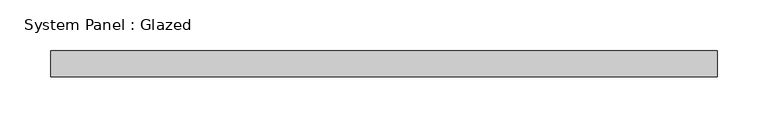
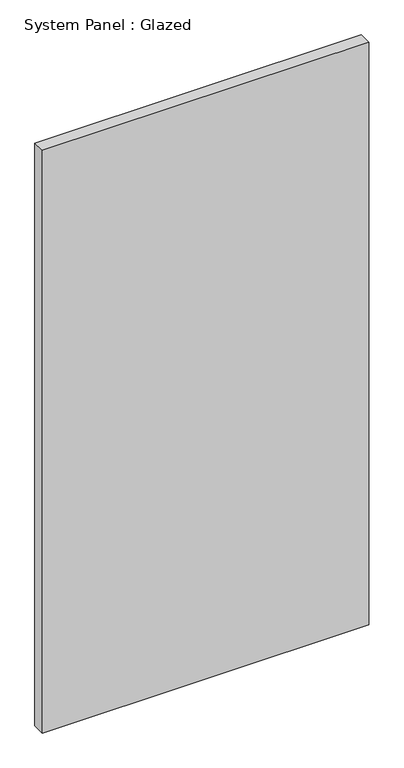
"""IFC4 building model written with IfcOpenShell, lengths in millimetres: plate geometry, System Panel : Glazed."""

from ifc_helpers import new_model, si_unit, origin, origin_with_axes, place, context, project, spatial, polyline, outline, extrude, source, transform, mapped, element, save


def system_panel_glazed_2a0e46e6(model_context):
    return source(origin(), model_context, "Body", "SweptSolid", [
        extrude(outline(polyline([(328.210424, 19.05), (-328.210424, 19.05), (-328.210424, 44.45), (328.210424, 44.45), (328.210424, 19.05)])), origin_with_axes(), (0.0, 0.0, 1.0), 1238.4610041),
    ])


if __name__ == "__main__":
    model = new_model("IFC4")
    model_context = context("Model", 3, world=origin())
    ifc_project = project(units=[si_unit("LENGTHUNIT", "METRE", prefix="MILLI")], contexts=[model_context])
    site = spatial("IfcSite", under=ifc_project)
    building = spatial("IfcBuilding", under=site)
    placement = place(None, origin())
    system_panel_glazed_shape = system_panel_glazed_2a0e46e6(model_context)
    element("IfcPlate", 1, ObjectType="System Panel : Glazed", at=placement, inside=building, context=model_context, shape_type="MappedRepresentation", body=[
        mapped(system_panel_glazed_shape, transform((0.0, 0.0, 0.0), x_axis=(1.0, 0.0, 0.0), y_axis=(0.0, 1.0, 0.0), z_axis=(0.0, 0.0, 1.0))),
    ])
    save(model, "model.ifc")

# Revit data of these elements
# Type "System Panel : Glazed"
#   Construction Type Id = "GSP4R"
#   Analytic Construction = "1/8 in Pilkington single glazing"
#   Visual Light Transmittance = 0.9
#   Solar Heat Gain Coefficient = 0.86
#   Heat Transfer Coefficient (U) = 1.18115 BTU/(h·ft²·°F)
#   Define Thermal Properties by = 1
# Element 1 (IfcPlate, "System Panel : Glazed")
#   Materials on its faces: "Glass"
# Materials
#   "Glass": class "Glass", colour RGB 0 128 192, transparency 0.75, Description = "Soda Lime Glass", Cost = 0
